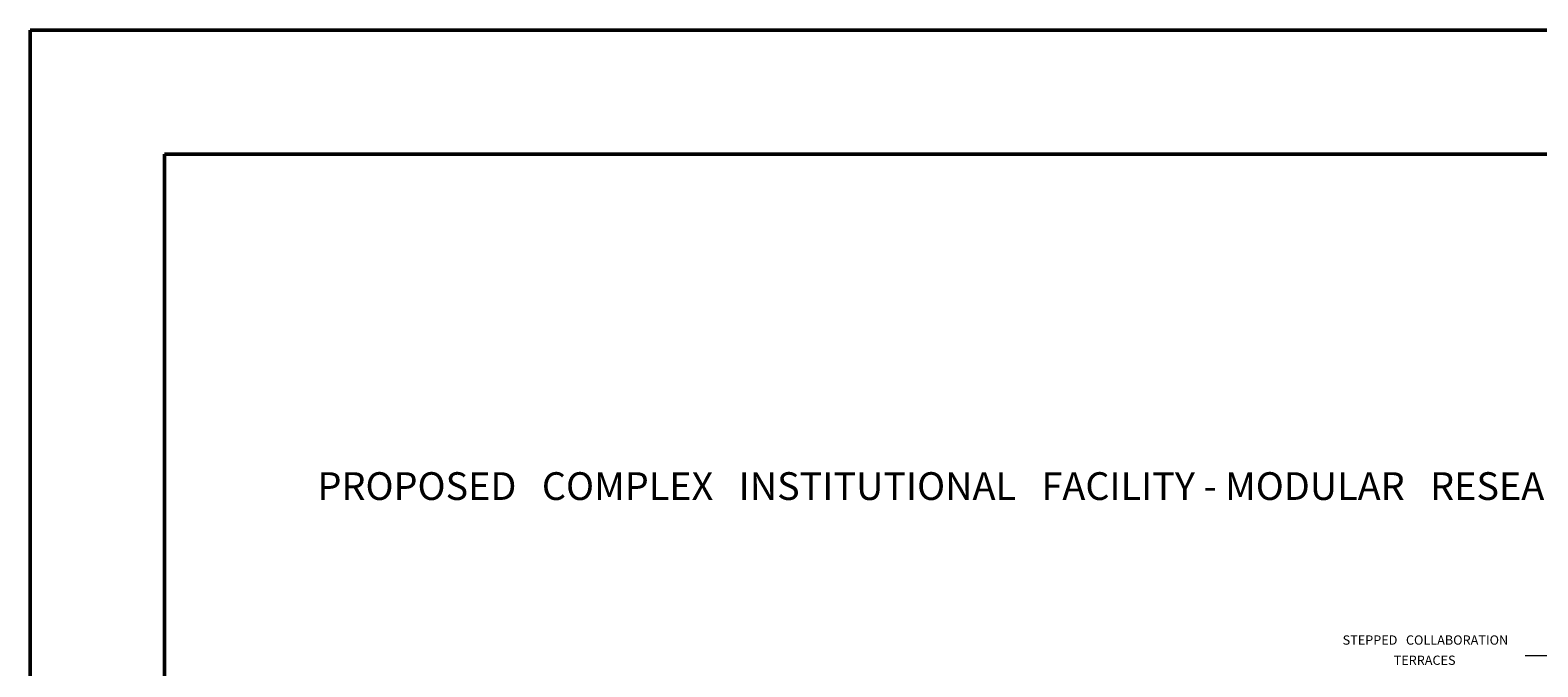
# Model space of a CAD drawing. Units: inches. Extents: x -1080 to 1950, y -1929 to 857.
# Tile 5 of 16: x -1080 to 294, y 276 to 857. Entities that reach past the tile are written whole.
import ezdxf

# ---------------------------------------------------------------- set-up
doc = ezdxf.new("R2010")
doc.units = ezdxf.units.IN
doc.header["$MEASUREMENT"] = 0
for name, color, linetype, lineweight in [('A-ANNO-SYMB', 2, 'Continuous', 18), ('A-ANNO-TEXT', 7, 'Continuous', 25), ('A-ANNO-TTLB', 7, 'Continuous', 50)]:
    doc.layers.add(name, color=color, linetype=linetype, lineweight=lineweight)
doc.styles.get("Standard").update_dxf_attribs({"font": 'arial.ttf'})

msp = doc.modelspace()

# ---------------------------------------------------------------- linework, layer by layer
at = {"layer": 'A-ANNO-SYMB'}
msp.add_line((314.1, 286.2), (282.4, 286.2), dxfattribs=at)
at = {"layer": 'A-ANNO-TTLB'}
for points in [[(-1080.1, 856.5), (1950.4, 856.5), (1950.4, -1929), (-1080.1, -1929)], [(-957.6, 743.5), (1813.4, 743.5), (1813.4, -1770.5), (-957.6, -1770.5)]]:
    msp.add_lwpolyline(points, close=True, dxfattribs=at)

# ---------------------------------------------------------------- texts
at = {"layer": 'A-ANNO-TEXT'}
for s, height, p in [('PROPOSED   COMPLEX   INSTITUTIONAL   FACILITY - MODULAR   RESEARCH   AND   INNOVATION   AXIS   ( CONCEPTUAL   ONLY - NO   DIMENSIONS )', 25.272, (-818.2, 428.4)), ('STEPPED   COLLABORATION', 8.461, (116, 296.5)), ('TERRACES', 8.46, (162.5, 278.1))]:
    msp.add_text(s, height=height, dxfattribs=at).set_placement(p)

doc.saveas('drawing.dxf')
